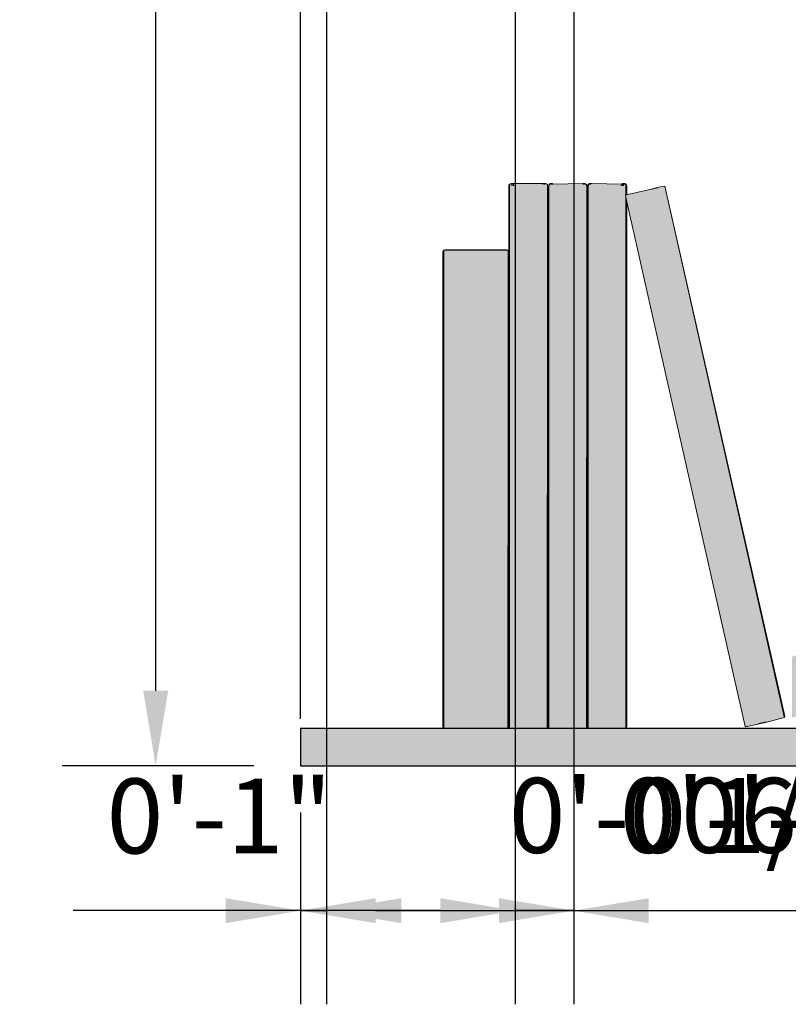
# Model space of a CAD drawing. Units: millimetres. Extents: x 7894 to 8038, y 6851 to 6951.
# Tile 16 of 49: x 7936.33 to 7946.6, y 6903.29 to 6916.43. Entities that reach past the tile are written whole.
import ezdxf

# ---------------------------------------------------------------- set-up
doc = ezdxf.new("R2010")
doc.units = ezdxf.units.MM
for name, color, linetype, lineweight in [('A-ANNO-DIMS', 2, 'Continuous', 18), ('A-FURN-BOOK', 8, 'Continuous', 13), ('A-FURN-SHLF', 7, 'Continuous', 30)]:
    doc.layers.add(name, color=color, linetype=linetype, lineweight=lineweight)
doc.layers.add('A-FURN-PATT', color=32, linetype='Continuous', lineweight=9, true_color=0xcd6928)
doc.styles.get("Standard").update_dxf_attribs({"font": 'arial.ttf'})
doc.dimstyles.new('ISO-25', dxfattribs={"dimtxt": 1, "dimasz": 1, "dimexe": 1.25, "dimexo": 0.625, "dimtad": 1, "dimdec": 0, "dimlunit": 4, "dimtxsty": 'Standard', "dimcen": 2.5, "dimclrt": 1, "dimadec": 0, "dimazin": 0, "dimtfac": 1, "dimtdec": 0, "dimtmove": 0, "dimatfit": 3, "dimfxl": 1, "dimarcsym": 0})

# ---------------------------------------------------------------- blocks, each defined once
blk = doc.blocks.new('*D23')
at = {"layer": 'A-ANNO-DIMS', "color": 0, "lineweight": -2, "transparency": 16777216}
for p, q in [((7940.089, 6907.098), (7940.089, 6947.793)), ((7971.936, 6928.989), (7971.936, 6947.793)), ((7941.089, 6946.543), (7970.936, 6946.543))]:
    blk.add_line(p, q, dxfattribs=at)
at = {"layer": 'A-ANNO-DIMS', "color": 0, "transparency": 16777216}
for points in [[(7941.089, 6946.709), (7941.089, 6946.376), (7940.089, 6946.543)], [(7970.936, 6946.709), (7970.936, 6946.376), (7971.936, 6946.543)]]:
    blk.add_solid(points, dxfattribs=at)
at = {"layer": 'Defpoints', "color": 0, "transparency": 16777216}
for p in [(7971.936, 6946.543), (7971.936, 6928.364), (7940.089, 6906.473)]:
    blk.add_point(p, dxfattribs=at)
at = {"layer": 'A-ANNO-DIMS', "color": 1, "transparency": 16777216, "insert": (7956.012, 6947.678), "char_height": 1, "attachment_point": 5}
blk.add_mtext('2\'-8"', dxfattribs=at)
blk = doc.blocks.new('*D24')
at = {"layer": 'A-ANNO-DIMS', "color": 0, "lineweight": -2, "transparency": 16777216}
for p, q in [((7953.341, 6944.606), (7936.902, 6944.606)), ((7938.152, 6907.473), (7938.152, 6943.606)), ((7939.464, 6906.473), (7936.902, 6906.473))]:
    blk.add_line(p, q, dxfattribs=at)
at = {"layer": 'A-ANNO-DIMS', "color": 0, "transparency": 16777216}
for points in [[(7937.986, 6943.606), (7938.319, 6943.606), (7938.152, 6944.606)], [(7937.986, 6907.473), (7938.319, 6907.473), (7938.152, 6906.473)]]:
    blk.add_solid(points, dxfattribs=at)
at = {"layer": 'Defpoints', "color": 0, "transparency": 16777216}
for p in [(7938.152, 6944.606), (7953.966, 6944.606), (7940.089, 6906.473)]:
    blk.add_point(p, dxfattribs=at)
at = {"layer": 'A-ANNO-DIMS', "color": 1, "transparency": 16777216, "insert": (7937.016, 6925.539), "char_height": 1, "attachment_point": 5, "rotation": 90}
blk.add_mtext('3\'-2"', dxfattribs=at)
blk = doc.blocks.new('*D25')
at = {"layer": 'A-ANNO-DIMS', "color": 0, "lineweight": -2, "transparency": 16777216}
for p, q in [((7940.089, 6905.848), (7940.089, 6903.287)), ((7964.341, 6905.848), (7964.341, 6903.287)), ((7941.089, 6904.537), (7963.341, 6904.537))]:
    blk.add_line(p, q, dxfattribs=at)
at = {"layer": 'A-ANNO-DIMS', "color": 0, "transparency": 16777216}
for points in [[(7941.089, 6904.703), (7941.089, 6904.37), (7940.089, 6904.537)], [(7963.341, 6904.703), (7963.341, 6904.37), (7964.341, 6904.537)]]:
    blk.add_solid(points, dxfattribs=at)
at = {"layer": 'Defpoints', "color": 0, "transparency": 16777216}
for p in [(7940.089, 6906.473), (7964.341, 6906.473), (7964.341, 6904.537)]:
    blk.add_point(p, dxfattribs=at)
at = {"layer": 'A-ANNO-DIMS', "color": 1, "transparency": 16777216, "insert": (7952.215, 6905.679), "char_height": 1, "attachment_point": 5}
blk.add_mtext('2\'-0 1/2"', dxfattribs=at)
blk = doc.blocks.new('*D29')
at = {"layer": 'A-ANNO-DIMS', "color": 0, "lineweight": -2, "transparency": 16777216}
for p, q in [((7940.435, 6923.814), (7940.435, 6903.287)), ((7943.737, 6918.095), (7943.737, 6903.287)), ((7941.435, 6904.537), (7942.737, 6904.537)), ((7943.737, 6904.537), (7950.975, 6904.537))]:
    blk.add_line(p, q, dxfattribs=at)
at = {"layer": 'A-ANNO-DIMS', "color": 0, "transparency": 16777216}
for points in [[(7941.435, 6904.703), (7941.435, 6904.37), (7940.435, 6904.537)], [(7942.737, 6904.703), (7942.737, 6904.37), (7943.737, 6904.537)]]:
    blk.add_solid(points, dxfattribs=at)
at = {"layer": 'Defpoints', "color": 0, "transparency": 16777216}
for p in [(7940.435, 6924.439), (7943.737, 6918.72), (7943.737, 6904.537)]:
    blk.add_point(p, dxfattribs=at)
at = {"layer": 'A-ANNO-DIMS', "color": 1, "transparency": 16777216, "insert": (7947.856, 6905.679), "char_height": 1, "attachment_point": 5}
blk.add_mtext('0\'-3 1/2"', dxfattribs=at)
blk = doc.blocks.new('*D32')
at = {"layer": 'A-ANNO-DIMS', "color": 0, "lineweight": -2, "transparency": 16777216}
for p, q in [((7943.737, 6918.095), (7943.737, 6903.287)), ((7950.34, 6918.095), (7950.34, 6903.287)), ((7944.737, 6904.537), (7949.34, 6904.537))]:
    blk.add_line(p, q, dxfattribs=at)
at = {"layer": 'A-ANNO-DIMS', "color": 0, "transparency": 16777216}
for points in [[(7944.737, 6904.703), (7944.737, 6904.37), (7943.737, 6904.537)], [(7949.34, 6904.703), (7949.34, 6904.37), (7950.34, 6904.537)]]:
    blk.add_solid(points, dxfattribs=at)
at = {"layer": 'Defpoints', "color": 0, "transparency": 16777216}
for p in [(7943.737, 6918.72), (7950.34, 6918.72), (7950.34, 6904.537)]:
    blk.add_point(p, dxfattribs=at)
at = {"layer": 'A-ANNO-DIMS', "color": 1, "transparency": 16777216, "insert": (7947.038, 6905.679), "char_height": 1, "attachment_point": 5}
blk.add_mtext('0\'-6 1/2"', dxfattribs=at)
blk = doc.blocks.new('*D33')
at = {"layer": 'A-ANNO-DIMS', "color": 0, "lineweight": -2, "transparency": 16777216}
for p, q in [((7940.435, 6923.814), (7940.435, 6903.287)), ((7940.089, 6905.848), (7940.089, 6903.287)), ((7939.089, 6904.537), (7938.089, 6904.537)), ((7940.089, 6904.537), (7940.435, 6904.537)), ((7941.435, 6904.537), (7948.673, 6904.537))]:
    blk.add_line(p, q, dxfattribs=at)
at = {"layer": 'A-ANNO-DIMS', "color": 0, "transparency": 16777216}
for points in [[(7939.089, 6904.703), (7939.089, 6904.37), (7940.089, 6904.537)], [(7941.435, 6904.703), (7941.435, 6904.37), (7940.435, 6904.537)]]:
    blk.add_solid(points, dxfattribs=at)
at = {"layer": 'Defpoints', "color": 0, "transparency": 16777216}
for p in [(7940.435, 6924.439), (7940.089, 6906.473), (7940.435, 6904.537)]:
    blk.add_point(p, dxfattribs=at)
at = {"layer": 'A-ANNO-DIMS', "color": 1, "transparency": 16777216, "insert": (7945.554, 6905.679), "char_height": 1, "attachment_point": 5}
blk.add_mtext('0\'-0 1/2"', dxfattribs=at)
blk = doc.blocks.new('*D35')
at = {"layer": 'A-ANNO-DIMS', "color": 0, "lineweight": -2, "transparency": 16777216}
for p, q in [((7942.957, 6936.255), (7942.957, 6903.287)), ((7943.737, 6929.533), (7943.737, 6903.287)), ((7941.957, 6904.537), (7937.049, 6904.537)), ((7943.737, 6904.537), (7942.957, 6904.537)), ((7944.737, 6904.537), (7945.737, 6904.537))]:
    blk.add_line(p, q, dxfattribs=at)
at = {"layer": 'A-ANNO-DIMS', "color": 0, "transparency": 16777216}
for points in [[(7941.957, 6904.703), (7941.957, 6904.37), (7942.957, 6904.537)], [(7944.737, 6904.703), (7944.737, 6904.37), (7943.737, 6904.537)]]:
    blk.add_solid(points, dxfattribs=at)
at = {"layer": 'Defpoints', "color": 0, "transparency": 16777216}
for p in [(7942.957, 6936.88), (7943.737, 6930.158), (7942.957, 6904.537)]:
    blk.add_point(p, dxfattribs=at)
at = {"layer": 'A-ANNO-DIMS', "color": 1, "transparency": 16777216, "insert": (7939.003, 6905.672), "char_height": 1, "attachment_point": 5}
blk.add_mtext('0\'-1"', dxfattribs=at)

msp = doc.modelspace()

# ---------------------------------------------------------------- hatches: boundary and pattern name
at = {"layer": 'A-FURN-PATT'}
h = msp.add_hatch(color=256, dxfattribs=at)
h.dxf.hatch_style = 1
h.paths.add_polyline_path([(7942.841, 6913.363), (7942.859, 6913.356), (7942.868, 6913.356), (7942.868, 6914.213), (7942.876, 6914.238), (7942.881, 6914.238), (7942.902, 6914.246), (7943.366, 6914.246), (7943.384, 6914.238), (7943.386, 6914.238), (7943.386, 6914.213), (7943.385, 6913.231), (7943.394, 6906.995), (7943.387, 6906.973), (7943.403, 6906.973), (7943.403, 6906.995), (7943.403, 6908.437), (7943.394, 6914.213), (7943.417, 6914.238), (7943.42, 6914.246), (7943.455, 6914.246), (7943.46, 6914.238), (7943.861, 6914.245), (7943.861, 6914.246), (7943.862, 6914.245), (7943.887, 6914.246), (7943.894, 6914.24), (7943.91, 6914.238), (7943.921, 6914.213), (7943.929, 6914.238), (7943.932, 6914.238), (7943.945, 6914.24), (7943.949, 6914.246), (7943.98, 6914.245), (7943.981, 6914.246), (7943.982, 6914.245), (7944.374, 6914.238), (7944.388, 6914.246), (7944.42, 6914.246), (7944.434, 6914.238), (7944.439, 6914.238), (7944.448, 6914.213), (7944.448, 6914.103), (7944.462, 6914.099), (7944.736, 6914.161), (7944.892, 6914.201), (7944.954, 6914.21), (7944.955, 6914.21), (7946.556, 6907.133), (7946.553, 6907.112), (7946.553, 6907.115), (7946.499, 6907.103), (7946.334, 6907.06), (7946.028, 6906.991), (7945.673, 6908.571), (7944.448, 6914.001), (7944.448, 6906.995), (7944.44, 6906.973), (7947.037, 6906.973), (7964.341, 6906.973), (7964.341, 6906.473), (7947.037, 6906.473), (7940.089, 6906.473), (7940.089, 6906.973), (7941.995, 6906.973), (7941.99, 6906.99), (7941.99, 6913.335), (7941.997, 6913.357), (7942.003, 6913.357), (7942.017, 6913.363), (7942.037, 6913.363), (7942.038, 6913.363), (7942.048, 6913.356), (7942.814, 6913.356), (7942.816, 6913.356), (7942.835, 6913.356)])
h.paths.add_polyline_path([(7942.86, 6913.02), (7942.861, 6913.335), (7942.868, 6906.995), (7942.876, 6906.976), (7942.876, 6906.99), (7942.881, 6914.238), (7942.876, 6914.232), (7942.876, 6914.218), (7942.881, 6906.965), (7942.878, 6906.97), (7942.876, 6906.97), (7942.857, 6906.97), (7942.861, 6911.855)], flags=16)
h.paths.add_polyline_path([(7942.861, 6911.855), (7942.868, 6906.995), (7942.869, 6906.992), (7942.868, 6906.99), (7942.862, 6906.97), (7942.86, 6906.97), (7942.857, 6906.97), (7942, 6906.97), (7941.998, 6906.97), (7941.996, 6906.97), (7941.99, 6906.99), (7941.998, 6906.97), (7942, 6906.97), (7942.86, 6906.97), (7942.862, 6906.975)], flags=16)
h.paths.add_polyline_path([(7942.023, 6913.356), (7942.017, 6913.363), (7942.037, 6913.363), (7942.038, 6913.363), (7942.037, 6913.361), (7942.037, 6913.356)], flags=16)
h.paths.add_polyline_path([(7942.037, 6913.363), (7942.017, 6913.363), (7942.02, 6913.36)], flags=0)
h.paths.add_polyline_path([(7942.035, 6913.356), (7942.037, 6913.356), (7942.037, 6913.361)], flags=0)
h.paths.add_polyline_path([(7943.929, 6906.976), (7943.921, 6906.995), (7943.929, 6906.97)], flags=0)
h.paths.add_polyline_path([(7943.913, 6914.213), (7943.898, 6914.238), (7943.894, 6914.24), (7943.883, 6914.242), (7943.878, 6914.237), (7943.876, 6914.238), (7943.879, 6914.238), (7943.887, 6914.246), (7943.862, 6914.245), (7943.861, 6914.245), (7943.861, 6914.246), (7943.862, 6914.245), (7943.887, 6914.246), (7943.894, 6914.24), (7943.898, 6914.238), (7943.91, 6914.218), (7943.913, 6914.217), (7943.908, 6906.97), (7943.91, 6906.97), (7943.921, 6914.213), (7943.929, 6914.238), (7943.932, 6914.238), (7943.945, 6914.24), (7943.949, 6914.246), (7943.98, 6914.245), (7943.981, 6914.246), (7943.982, 6914.245), (7944.374, 6914.238), (7944.388, 6914.246), (7944.42, 6914.246), (7944.434, 6914.238), (7944.439, 6914.238), (7944.439, 6914.218), (7944.434, 6914.094), (7944.448, 6914.1), (7944.451, 6914.102), (7944.462, 6914.099), (7944.434, 6914.093), (7944.429, 6914.091), (7944.434, 6914.069), (7944.448, 6914.001), (7944.434, 6914.065), (7944.435, 6906.97), (7944.437, 6906.97), (7944.439, 6906.976), (7944.439, 6906.97), (7943.931, 6906.97), (7943.913, 6906.97), (7943.908, 6906.97)], flags=16)
h.paths.add_polyline_path([(7943.921, 6914.213), (7943.929, 6914.238), (7943.932, 6914.238), (7943.945, 6914.24), (7943.949, 6914.246), (7943.98, 6914.245), (7943.981, 6914.246), (7943.982, 6914.245), (7944.374, 6914.238), (7944.388, 6914.246), (7944.42, 6914.246), (7944.432, 6914.239), (7944.425, 6914.238), (7944.404, 6914.238), (7944.403, 6914.214), (7944.403, 6914.238), (7944.402, 6914.238), (7944.39, 6914.238), (7944.375, 6914.238), (7944.374, 6914.238), (7943.982, 6914.245), (7943.949, 6914.246), (7943.945, 6914.24), (7943.929, 6914.213), (7943.931, 6906.972), (7943.931, 6906.97), (7943.929, 6906.97), (7943.929, 6906.976), (7943.929, 6914.213), (7943.944, 6914.238), (7943.932, 6914.238)], flags=0)
h.paths.add_polyline_path([(7942.881, 6914.238), (7942.878, 6914.236), (7942.88, 6914.24), (7942.885, 6914.239)], flags=17)
h.paths.add_polyline_path([(7944.412, 6914.242), (7944.41, 6914.241), (7944.412, 6914.242)], flags=0)
h.paths.add_polyline_path([(7944.388, 6914.238), (7944.388, 6914.246), (7944.409, 6914.241), (7944.41, 6914.241), (7944.404, 6914.237), (7944.39, 6914.245), (7944.39, 6914.238)], flags=0)
h.paths.add_polyline_path([(7963.136, 6906.953), (7963.14, 6906.953), (7963.143, 6906.958)], flags=16)
h.paths.add_polyline_path([(7954.398, 6907.39), (7954.397, 6907.395), (7954.398, 6907.401), (7954.397, 6907.567), (7954.398, 6907.598), (7954.399, 6907.769), (7954.398, 6907.799), (7954.399, 6907.876), (7954.399, 6907.904), (7954.394, 6907.908), (7954.402, 6907.905), (7954.4, 6907.93), (7954.399, 6907.931), (7954.384, 6907.943), (7946.675, 6907.943), (7946.653, 6907.923), (7946.653, 6907.913), (7946.653, 6907.769), (7946.653, 6907.401), (7946.653, 6907.118), (7946.657, 6907.122), (7946.656, 6907.115), (7946.657, 6907.113), (7946.667, 6907.121), (7946.752, 6907.121), (7946.91, 6907.121), (7954.3, 6907.121), (7954.39, 6907.121), (7954.392, 6907.119), (7954.399, 6907.121), (7954.399, 6907.138), (7954.398, 6907.216), (7954.399, 6907.241)], flags=17)
h.paths.add_polyline_path([(7954.3, 6907.121), (7954.3, 6907.114), (7946.911, 6907.113), (7946.752, 6907.114), (7946.752, 6907.121), (7946.667, 6907.121), (7946.653, 6907.111), (7946.653, 6907.118), (7946.657, 6907.122), (7946.656, 6907.115), (7946.657, 6907.113), (7946.667, 6907.121), (7946.752, 6907.121), (7946.91, 6907.121)], flags=17)
h.paths.add_polyline_path([(7954.398, 6907.905), (7954.394, 6907.908), (7954.4, 6907.906), (7954.401, 6907.919), (7954.402, 6907.905), (7954.405, 6907.907), (7954.404, 6907.905), (7954.403, 6907.897), (7954.402, 6907.901), (7954.4, 6907.903), (7954.4, 6907.902), (7954.399, 6907.902), (7954.399, 6907.904)], flags=17)
h = msp.add_hatch(color=256, dxfattribs=at)
h.dxf.hatch_style = 1
h.paths.add_polyline_path([(7943.385, 6913.231), (7943.386, 6914.213), (7943.384, 6914.237), (7943.337, 6914.246), (7942.926, 6914.246), (7942.926, 6914.214), (7942.881, 6914.212), (7942.881, 6906.973), (7943.381, 6906.973)])
h.paths.add_polyline_path([(7943.384, 6906.97), (7943.386, 6906.976), (7943.386, 6906.97)])
h = msp.add_hatch(color=256, dxfattribs=at)
h.dxf.hatch_style = 1
h.paths.add_polyline_path([(7943.913, 6914.213), (7943.898, 6914.238), (7943.894, 6914.24), (7943.883, 6914.242), (7943.879, 6914.238), (7943.876, 6914.238), (7943.863, 6914.238), (7943.862, 6914.245), (7943.46, 6914.238), (7943.417, 6914.237), (7943.414, 6914.234), (7943.403, 6914.213), (7943.403, 6908.437), (7943.403, 6906.995), (7943.407, 6906.973), (7943.908, 6906.973)])
h.paths.add_polyline_path([(7943.403, 6906.995), (7943.407, 6906.973), (7943.408, 6906.97), (7943.403, 6906.97)])
h = msp.add_hatch(color=256, dxfattribs=at)
h.dxf.hatch_style = 1
h.paths.add_polyline_path([(7944.434, 6914.069), (7944.429, 6914.092), (7944.434, 6914.094), (7944.434, 6914.236), (7944.425, 6914.238), (7944.404, 6914.238), (7944.388, 6914.238), (7944.388, 6914.238), (7944.375, 6914.238), (7944.374, 6914.238), (7943.982, 6914.245), (7943.949, 6914.246), (7943.945, 6914.24), (7943.929, 6914.213), (7943.931, 6906.973), (7944.435, 6906.973)])
h.paths.add_polyline_path([(7944.404, 6914.238), (7944.404, 6914.235), (7944.407, 6914.238)], flags=17)
h.paths.add_polyline_path([(7944.388, 6914.238), (7944.39, 6914.238), (7944.405, 6914.238), (7944.411, 6914.242), (7944.439, 6914.238), (7944.439, 6914.234), (7944.425, 6914.238), (7944.404, 6914.238), (7944.388, 6914.238), (7944.388, 6914.238), (7944.374, 6914.238), (7944.374, 6914.238), (7944.375, 6914.238)])

# ---------------------------------------------------------------- linework, layer by layer
at = {"layer": 'A-FURN-BOOK'}
for p, q in [((7942.868, 6914.213), (7942.876, 6914.238)), ((7942.876, 6914.232), (7942.868, 6914.213)), ((7942.868, 6906.995), (7942.868, 6914.213)), ((7942.876, 6914.238), (7942.878, 6914.238)), ((7942.876, 6914.238), (7942.876, 6914.232)), ((7942.878, 6914.238), (7942.876, 6914.232)), ((7942.876, 6914.232), (7942.876, 6914.218)), ((7942.878, 6914.238), (7942.881, 6914.238)), ((7942.881, 6914.238), (7942.885, 6914.239)), ((7942.881, 6914.238), (7942.881, 6906.97)), ((7942.885, 6914.239), (7942.902, 6914.246)), ((7942.894, 6914.24), (7942.885, 6914.239)), ((7942.885, 6914.239), (7942.891, 6914.238)), ((7942.895, 6914.241), (7942.894, 6914.24)), ((7943.366, 6914.246), (7942.902, 6914.246)), ((7942.911, 6914.214), (7942.91, 6914.238)), ((7942.912, 6914.214), (7942.912, 6914.238)), ((7942.926, 6914.238), (7942.929, 6914.214)), ((7942.926, 6914.214), (7942.926, 6914.238)), ((7942.926, 6914.238), (7942.927, 6914.214)), ((7942.934, 6914.238), (7942.936, 6914.215)), ((7943.32, 6914.236), (7943.32, 6914.238)), ((7943.324, 6914.238), (7943.32, 6914.238)), ((7943.334, 6914.236), (7943.334, 6914.238)), ((7943.336, 6914.238), (7943.336, 6914.237)), ((7943.35, 6914.238), (7943.336, 6914.238)), ((7943.361, 6914.242), (7943.384, 6914.238)), ((7943.366, 6914.246), (7943.384, 6914.238)), ((7943.386, 6914.213), (7943.384, 6914.238)), ((7943.386, 6914.238), (7943.384, 6914.238)), ((7943.384, 6914.238), (7943.384, 6914.238)), ((7943.386, 6914.213), (7943.385, 6913.231)), ((7943.386, 6914.213), (7943.386, 6914.238)), ((7943.394, 6906.995), (7943.386, 6914.213)), ((7943.394, 6914.213), (7943.414, 6914.234)), ((7943.403, 6908.437), (7943.394, 6914.213)), ((7943.394, 6914.213), (7943.403, 6906.995)), ((7943.403, 6914.213), (7943.414, 6914.234)), ((7943.403, 6908.437), (7943.403, 6914.213)), ((7943.414, 6914.234), (7943.417, 6914.238)), ((7943.417, 6914.238), (7943.42, 6914.246)), ((7943.417, 6914.238), (7943.438, 6914.242)), ((7943.455, 6914.246), (7943.42, 6914.246)), ((7943.433, 6914.238), (7943.452, 6914.238)), ((7943.453, 6914.239), (7943.452, 6914.238)), ((7943.452, 6914.238), (7943.46, 6914.238)), ((7943.46, 6914.238), (7943.455, 6914.246)), ((7943.46, 6914.238), (7943.861, 6914.245)), ((7943.859, 6914.238), (7943.863, 6914.238)), ((7943.862, 6914.245), (7943.861, 6914.246)), ((7943.861, 6914.246), (7943.861, 6914.245)), ((7943.862, 6914.245), (7943.887, 6914.246)), ((7943.863, 6914.238), (7943.863, 6914.239)), ((7943.876, 6914.238), (7943.863, 6914.238)), ((7943.876, 6914.238), (7943.87, 6914.241)), ((7943.879, 6914.238), (7943.876, 6914.238)), ((7943.878, 6914.243), (7943.883, 6914.242)), ((7943.883, 6914.242), (7943.879, 6914.238)), ((7943.887, 6914.246), (7943.883, 6914.242)), ((7943.883, 6914.242), (7943.894, 6914.24)), ((7943.887, 6914.246), (7943.894, 6914.24)), ((7943.894, 6914.24), (7943.898, 6914.238)), ((7943.894, 6914.24), (7943.91, 6914.238)), ((7943.91, 6914.218), (7943.898, 6914.238)), ((7943.908, 6906.97), (7943.913, 6914.213)), ((7943.921, 6914.213), (7943.91, 6914.238)), ((7943.91, 6914.218), (7943.91, 6914.218)), ((7943.913, 6914.213), (7943.91, 6914.218)), ((7943.91, 6906.97), (7943.921, 6914.213)), ((7943.913, 6906.97), (7943.921, 6914.213)), ((7943.921, 6914.213), (7943.929, 6914.238)), ((7943.932, 6914.238), (7943.921, 6914.213)), ((7943.921, 6906.995), (7943.921, 6914.213)), ((7943.921, 6914.213), (7943.929, 6906.976)), ((7943.929, 6914.238), (7943.932, 6914.238)), ((7943.929, 6914.213), (7943.944, 6914.238)), ((7943.931, 6906.972), (7943.929, 6914.213)), ((7943.932, 6914.238), (7943.945, 6914.24)), ((7943.944, 6914.238), (7943.932, 6914.238)), ((7943.944, 6914.238), (7943.945, 6914.24)), ((7943.96, 6914.238), (7943.944, 6914.238)), ((7943.945, 6914.24), (7943.949, 6914.246)), ((7943.945, 6914.24), (7943.955, 6914.241)), ((7943.98, 6914.245), (7943.949, 6914.246)), ((7943.979, 6914.237), (7943.979, 6914.238)), ((7943.981, 6914.246), (7943.98, 6914.245)), ((7943.98, 6914.245), (7943.982, 6914.245)), ((7943.981, 6914.246), (7943.982, 6914.245)), ((7943.981, 6914.236), (7943.981, 6914.238)), ((7943.982, 6914.245), (7944.374, 6914.238)), ((7943.993, 6914.236), (7943.993, 6914.238)), ((7944.374, 6914.238), (7944.373, 6914.215)), ((7944.374, 6914.238), (7944.375, 6914.238)), ((7944.375, 6914.238), (7944.388, 6914.246)), ((7944.375, 6914.238), (7944.388, 6914.238)), ((7944.388, 6914.238), (7944.387, 6914.214)), ((7944.388, 6914.246), (7944.39, 6914.238)), ((7944.402, 6914.238), (7944.388, 6914.246)), ((7944.388, 6914.246), (7944.42, 6914.246)), ((7944.388, 6914.246), (7944.388, 6914.238)), ((7944.388, 6914.246), (7944.409, 6914.241)), ((7944.412, 6914.242), (7944.388, 6914.246)), ((7944.388, 6914.238), (7944.39, 6914.238)), ((7944.39, 6914.238), (7944.389, 6914.214)), ((7944.39, 6914.238), (7944.39, 6914.214)), ((7944.39, 6914.238), (7944.402, 6914.238)), ((7944.402, 6914.238), (7944.404, 6914.238)), ((7944.402, 6914.238), (7944.403, 6914.238)), ((7944.403, 6914.214), (7944.403, 6914.238)), ((7944.403, 6914.214), (7944.404, 6914.238)), ((7944.403, 6914.238), (7944.404, 6914.238)), ((7944.404, 6914.238), (7944.425, 6914.238)), ((7944.404, 6914.238), (7944.405, 6914.238)), ((7944.405, 6914.238), (7944.409, 6914.241)), ((7944.409, 6914.241), (7944.41, 6914.241)), ((7944.41, 6914.241), (7944.412, 6914.242)), ((7944.41, 6914.241), (7944.425, 6914.238)), ((7944.412, 6914.242), (7944.42, 6914.246)), ((7944.432, 6914.239), (7944.412, 6914.242)), ((7944.412, 6914.242), (7944.412, 6914.242)), ((7944.432, 6914.239), (7944.42, 6914.246)), ((7944.425, 6914.238), (7944.432, 6914.239)), ((7944.434, 6914.238), (7944.432, 6914.239)), ((7944.434, 6914.238), (7944.434, 6914.094)), ((7944.439, 6914.238), (7944.434, 6914.238)), ((7944.439, 6914.238), (7944.448, 6914.213)), ((7944.439, 6914.218), (7944.439, 6914.238)), ((7944.448, 6914.213), (7944.448, 6914.1)), ((7944.462, 6914.099), (7944.736, 6914.161)), ((7944.736, 6914.161), (7944.892, 6914.201)), ((7944.736, 6914.161), (7944.863, 6914.189)), ((7944.954, 6914.21), (7944.892, 6914.201)), ((7944.955, 6914.21), (7944.954, 6914.21)), ((7944.954, 6914.21), (7946.551, 6907.127)), ((7946.556, 6907.133), (7944.955, 6914.21)), ((7944.429, 6914.091), (7944.434, 6914.094)), ((7944.429, 6914.091), (7944.434, 6914.093)), ((7944.434, 6914.069), (7944.429, 6914.091)), ((7944.434, 6914.094), (7944.448, 6914.1)), ((7944.462, 6914.099), (7944.434, 6914.093)), ((7944.434, 6914.094), (7944.434, 6914.093)), ((7944.434, 6914.069), (7944.434, 6914.065)), ((7944.434, 6914.065), (7944.435, 6906.97)), ((7944.448, 6914.001), (7944.434, 6914.065)), ((7944.451, 6914.102), (7944.448, 6914.1)), ((7944.448, 6914.1), (7944.448, 6914.098)), ((7944.451, 6914.102), (7944.462, 6914.099)), ((7944.448, 6914.001), (7945.673, 6908.571)), ((7944.448, 6914.001), (7944.448, 6906.995)), ((7942.003, 6913.357), (7942.017, 6913.363)), ((7942.017, 6913.363), (7942.037, 6913.363)), ((7942.02, 6913.36), (7942.017, 6913.363)), ((7942.02, 6913.36), (7942.037, 6913.363)), ((7942.032, 6913.356), (7942.037, 6913.361)), ((7942.035, 6913.356), (7942.037, 6913.361)), ((7942.038, 6913.363), (7942.037, 6913.363)), ((7942.037, 6913.361), (7942.037, 6913.363)), ((7942.037, 6913.356), (7942.037, 6913.361)), ((7942.037, 6913.361), (7942.048, 6913.356)), ((7942.048, 6913.356), (7942.038, 6913.363)), ((7942.038, 6913.363), (7942.841, 6913.363)), ((7942.822, 6913.356), (7942.841, 6913.363)), ((7942.841, 6913.363), (7942.835, 6913.356)), ((7942.841, 6913.363), (7942.859, 6913.356)), ((7941.99, 6913.335), (7941.996, 6913.356)), ((7941.996, 6913.351), (7941.99, 6913.335)), ((7941.99, 6906.99), (7941.99, 6913.335)), ((7941.996, 6913.356), (7941.998, 6913.356)), ((7941.996, 6913.356), (7941.996, 6913.351)), ((7941.998, 6913.356), (7941.996, 6913.351)), ((7941.996, 6913.351), (7941.996, 6913.339)), ((7941.998, 6913.356), (7942, 6913.356)), ((7942, 6913.356), (7942.003, 6913.357)), ((7942, 6906.97), (7942, 6913.356)), ((7942.003, 6913.357), (7942.02, 6913.36)), ((7942.023, 6913.356), (7942.003, 6913.357)), ((7942.023, 6913.356), (7942.02, 6913.36)), ((7942.023, 6913.356), (7942.032, 6913.356)), ((7942.035, 6913.356), (7942.032, 6913.356)), ((7942.035, 6913.356), (7942.037, 6913.356)), ((7942.048, 6913.356), (7942.037, 6913.356)), ((7942.814, 6913.356), (7942.048, 6913.356)), ((7942.816, 6913.356), (7942.814, 6913.356)), ((7942.822, 6913.356), (7942.816, 6913.356)), ((7942.822, 6913.356), (7942.833, 6913.356)), ((7942.833, 6913.356), (7942.835, 6913.356)), ((7942.834, 6913.356), (7942.833, 6913.356)), ((7942.835, 6913.356), (7942.834, 6913.356)), ((7942.835, 6913.356), (7942.837, 6913.356)), ((7942.837, 6913.356), (7942.859, 6913.356)), ((7942.861, 6913.356), (7942.859, 6913.356)), ((7942.861, 6913.335), (7942.859, 6913.356)), ((7942.861, 6913.335), (7942.86, 6913.02)), ((7942.861, 6913.335), (7942.861, 6913.356)), ((7942.868, 6906.995), (7942.861, 6913.335)), ((7943.385, 6913.231), (7943.381, 6906.97)), ((7943.385, 6913.231), (7943.394, 6906.995)), ((7942.86, 6913.02), (7942.861, 6911.855)), ((7942.861, 6911.855), (7942.857, 6906.97)), ((7942.861, 6911.855), (7942.868, 6906.995)), ((7942.862, 6906.975), (7942.861, 6911.855)), ((7945.673, 6908.571), (7946.027, 6906.997)), ((7946.028, 6906.997), (7945.673, 6908.571)), ((7943.403, 6906.995), (7943.403, 6908.437)), ((7946.037, 6906.993), (7946.334, 6907.06)), ((7946.209, 6907.038), (7946.29, 6907.056)), ((7946.334, 6907.06), (7946.29, 6907.056)), ((7946.499, 6907.103), (7946.334, 6907.06)), ((7946.499, 6907.103), (7946.553, 6907.115)), ((7946.554, 6907.115), (7946.551, 6907.127)), ((7946.551, 6907.127), (7946.553, 6907.115)), ((7946.554, 6907.115), (7946.553, 6907.115)), ((7946.556, 6907.133), (7946.554, 6907.115)), ((7941.996, 6906.97), (7941.99, 6906.99)), ((7941.99, 6906.99), (7941.996, 6906.974)), ((7941.996, 6906.974), (7941.996, 6906.97)), ((7941.996, 6906.974), (7941.998, 6906.97)), ((7941.996, 6906.97), (7941.998, 6906.97)), ((7941.998, 6906.97), (7942, 6906.97)), ((7942, 6906.97), (7942.857, 6906.97)), ((7942.857, 6906.97), (7942.86, 6906.97)), ((7942.86, 6906.97), (7942.862, 6906.975)), ((7942.86, 6906.97), (7942.862, 6906.97)), ((7942.868, 6906.99), (7942.862, 6906.97)), ((7942.862, 6906.975), (7942.868, 6906.99)), ((7942.862, 6906.97), (7942.862, 6906.975)), ((7942.862, 6906.97), (7942.876, 6906.97)), ((7942.876, 6906.97), (7942.868, 6906.995)), ((7942.868, 6906.995), (7942.876, 6906.976)), ((7942.868, 6906.99), (7942.868, 6906.995)), ((7942.876, 6906.99), (7942.876, 6906.976)), ((7942.876, 6906.976), (7942.876, 6906.97)), ((7942.876, 6906.976), (7942.878, 6906.97)), ((7942.878, 6906.97), (7942.876, 6906.97)), ((7942.878, 6906.97), (7942.881, 6906.97)), ((7943.381, 6906.97), (7942.881, 6906.97)), ((7943.381, 6906.97), (7943.384, 6906.97)), ((7943.384, 6906.97), (7943.386, 6906.976)), ((7943.386, 6906.97), (7943.384, 6906.97)), ((7943.394, 6906.995), (7943.386, 6906.97)), ((7943.386, 6906.976), (7943.394, 6906.995)), ((7943.386, 6906.97), (7943.386, 6906.976)), ((7943.386, 6906.97), (7943.403, 6906.97)), ((7943.403, 6906.995), (7943.403, 6906.97)), ((7943.403, 6906.995), (7943.405, 6906.984)), ((7943.403, 6906.97), (7943.405, 6906.97)), ((7943.405, 6906.97), (7943.405, 6906.984)), ((7943.405, 6906.984), (7943.408, 6906.97)), ((7943.405, 6906.97), (7943.408, 6906.97)), ((7943.408, 6906.97), (7943.908, 6906.97)), ((7943.91, 6906.97), (7943.908, 6906.97)), ((7943.91, 6906.97), (7943.913, 6906.97)), ((7943.913, 6906.97), (7943.929, 6906.97)), ((7943.929, 6906.97), (7943.921, 6906.995)), ((7943.921, 6906.995), (7943.929, 6906.976)), ((7943.929, 6906.976), (7943.929, 6906.97)), ((7943.929, 6906.976), (7943.931, 6906.972)), ((7943.931, 6906.97), (7943.929, 6906.97)), ((7943.931, 6906.97), (7943.931, 6906.972)), ((7944.435, 6906.97), (7943.931, 6906.97)), ((7944.435, 6906.97), (7944.437, 6906.97)), ((7944.437, 6906.97), (7944.439, 6906.976)), ((7944.439, 6906.97), (7944.437, 6906.97)), ((7944.448, 6906.995), (7944.439, 6906.97)), ((7944.439, 6906.976), (7944.448, 6906.995)), ((7944.439, 6906.97), (7944.439, 6906.976)), ((7946.027, 6906.997), (7946.028, 6906.997)), ((7946.037, 6906.993), (7946.028, 6906.997)), ((7946.037, 6906.993), (7946.036, 6906.999)), ((7946.037, 6906.993), (7946.057, 6907.002)), ((7946.209, 6907.038), (7946.207, 6907.037))]:
    msp.add_line(p, q, dxfattribs=at)
at = {"layer": 'A-FURN-SHLF'}
for p, q in [((7940.089, 6906.973), (7940.089, 6906.473)), ((7940.089, 6906.973), (7947.037, 6906.973)), ((7940.089, 6906.473), (7947.037, 6906.473))]:
    msp.add_line(p, q, dxfattribs=at)

# ---------------------------------------------------------------- dimensions: what is measured, and where the dimension line sits
at = {"layer": 'A-ANNO-DIMS'}
for base, p1, p2, picture, middle in [((7971.936, 6946.543), (7940.089, 6906.473), (7971.936, 6928.364), '*D23', (7956.012, 6947.678)), ((7942.957, 6904.537), (7943.737, 6930.158), (7942.957, 6936.88), '*D35', (7939.003, 6905.672)), ((7940.435, 6904.537), (7940.089, 6906.473), (7940.435, 6924.439), '*D33', (7945.554, 6905.679)), ((7943.737, 6904.537), (7940.435, 6924.439), (7943.737, 6918.72), '*D29', (7947.856, 6905.679)), ((7950.34, 6904.537), (7943.737, 6918.72), (7950.34, 6918.72), '*D32', (7947.038, 6905.679)), ((7964.341, 6904.537), (7940.089, 6906.473), (7964.341, 6906.473), '*D25', (7952.215, 6905.679))]:
    dim = msp.add_linear_dim(base=base, p1=p1, p2=p2, dimstyle='ISO-25', override={"dimdec": 1, "dimlfac": 1, "dimrnd": 0, "dimzin": 1, "dimdsep": 46, "dimlunit": 4, "dimfrac": 2}, dxfattribs=at)
    dim.commit()
    dim.dimension.update_dxf_attribs({"geometry": picture, "text_midpoint": middle})
dim = msp.add_linear_dim(base=(7938.152, 6944.606), p1=(7940.089, 6906.473), p2=(7953.966, 6944.606), angle=90, dimstyle='ISO-25', override={"dimdec": 1, "dimlfac": 1, "dimrnd": 0, "dimzin": 1, "dimdsep": 46, "dimlunit": 4, "dimfrac": 2}, dxfattribs=at)
dim.commit()
dim.dimension.update_dxf_attribs({"geometry": '*D24', "text_midpoint": (7937.016, 6925.539)})

doc.saveas('drawing.dxf')
